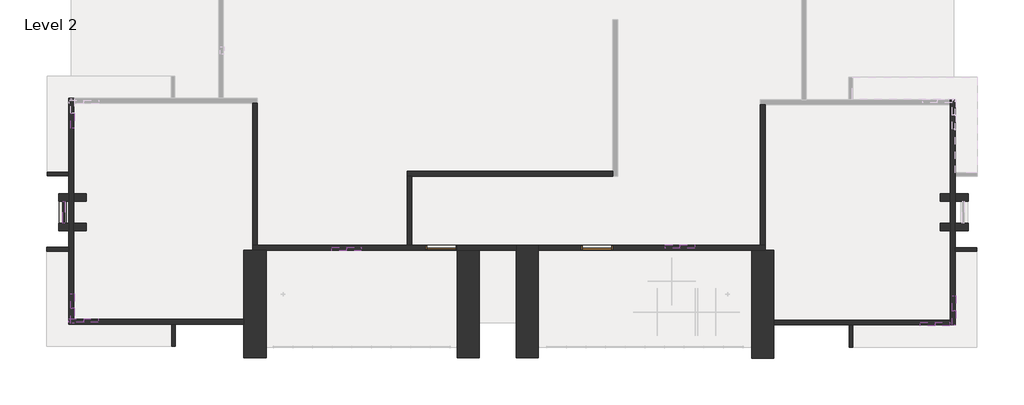
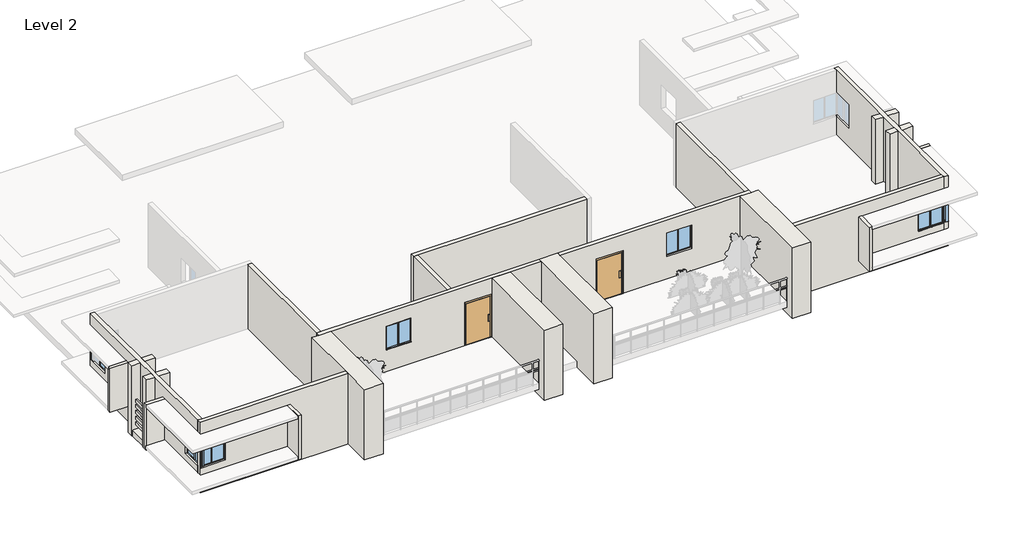
# One storey, part 1 of 4: 39 walls, 13 windows, 2 doors.
"""IFC4 building model written with IfcOpenShell, lengths in millimetres."""

from ifc_helpers import new_model, si_unit, frame, origin, place, context, project, spatial, polyline, outline, extrude, faceted_brep, transform, mapped, element, save
from components import door_15d3c954, window_20ff4747

model = new_model("IFC4")

# Units and contexts
model_context = context("Model", 3, world=origin())
ifc_project = project(units=[si_unit("LENGTHUNIT", "METRE", prefix="MILLI")], contexts=[model_context])

# Site, building, storey
site = spatial("IfcSite", under=ifc_project)
building = spatial("IfcBuilding", under=site)
storey = spatial("IfcBuildingStorey", under=building, Name="Level 2", Elevation=3048.0)

# Doors
placement = place(None, origin())
door_shape = door_15d3c954(model_context)
element("IfcDoor", 1, ObjectType="Door-Passage-Single-Flush-Dbl_Acting : 48\" x 96\"", at=placement, inside=storey, context=model_context, shape_type="MappedRepresentation", body=[
    mapped(door_shape, transform((7011.0520665, -5255.880811, 3657.6), x_axis=(-1.0, 0.0, 0.0), y_axis=(0.0, -1.0, 0.0), z_axis=(0.0, 0.0, 1.0))),
])
element("IfcDoor", 2, ObjectType="Door-Passage-Single-Flush-Dbl_Acting : 48\" x 96\"", at=placement, inside=storey, context=model_context, shape_type="MappedRepresentation", body=[
    mapped(door_shape, transform((559.4520665, -5255.1961695, 3657.6), x_axis=(-1.0, 0.0, 0.0), y_axis=(0.0, -1.0, 0.0), z_axis=(0.0, 0.0, 1.0))),
])

# Walls
element("IfcWall", 3, ObjectType="Generic - 1'", at=placement, inside=storey, context=model_context, shape_type="SweptSolid", body=[
    extrude(outline(polyline([(-14151.7972154, -3343.5294056), (-14680.5479335, -3343.5294056), (-14680.5479335, -3038.7294056), (-14151.7972154, -3038.7294056), (-14151.7972154, -3343.5294056)])), frame((0.0, 0.0, 3048.0), z_axis=(0.0, 0.0, 1.0), x_axis=(1.0, 0.0, 0.0)), (0.0, 0.0, 1.0), 3657.6),
])
element("IfcWall", 4, ObjectType="Generic - 1'", at=placement, inside=storey, context=model_context, shape_type="Brep", body=[
    faceted_brep([(-14883.7479335, -3038.7294056, 3048.0), (-15302.1394029, -3038.7294056, 3048.0), (-15302.1394029, -3038.7294056, 6705.6), (-14883.7479335, -3038.7294056, 6705.6), (-14883.7479335, -3343.5294056, 3048.0), (-14883.7479335, -3343.5294056, 6705.6), (-15302.1394029, -3343.5294056, 6705.6), (-15302.1394029, -3343.5294056, 3048.0), (-15277.0936682, -3343.5294056, 3048.0), (-14972.2936682, -3343.5294056, 3048.0)], [[[0, 1, 2, 3]], [[4, 5, 6, 7, 8, 9]], [[1, 0, 4, 9, 8, 7]], [[2, 1, 7, 6]], [[3, 2, 6, 5]], [[0, 3, 5, 4]]]),
])
element("IfcWall", 5, ObjectType="Generic - 1'", at=placement, inside=storey, context=model_context, shape_type="SweptSolid", body=[
    extrude(outline(polyline([(-14151.7972154, -4562.7294056), (-14680.5479335, -4562.7294056), (-14680.5479335, -4257.9294056), (-14151.7972154, -4257.9294056), (-14151.7972154, -4562.7294056)])), frame((0.0, 0.0, 3048.0), z_axis=(0.0, 0.0, 1.0), x_axis=(1.0, 0.0, 0.0)), (0.0, 0.0, 1.0), 3657.6),
])
element("IfcWall", 6, ObjectType="Generic - 1'", at=placement, inside=storey, context=model_context, shape_type="Brep", body=[
    faceted_brep([(-14883.7479335, -4257.9294056, 3048.0), (-14972.2936682, -4257.9294056, 3048.0), (-15277.0936682, -4257.9294056, 3048.0), (-15302.1394029, -4257.9294056, 3048.0), (-15302.1394029, -4257.9294056, 6705.6), (-14883.7479335, -4257.9294056, 6705.6), (-14883.7479335, -4562.7294056, 3048.0), (-14883.7479335, -4562.7294056, 6705.6), (-15302.1394029, -4562.7294056, 6705.6), (-15302.1394029, -4562.7294056, 3048.0)], [[[0, 1, 2, 3, 4, 5]], [[6, 7, 8, 9]], [[3, 2, 1, 0, 6, 9]], [[4, 3, 9, 8]], [[5, 4, 8, 7]], [[0, 5, 7, 6]]]),
])
element("IfcWall", 7, ObjectType="Generic - 1'", at=placement, inside=storey, context=model_context, shape_type="Brep", body=[
    faceted_brep([(21857.3520665, -3343.5294056, 3048.0), (22069.7857703, -3343.5294056, 3048.0), (22374.5857703, -3343.5294056, 3048.0), (22386.1027846, -3343.5294056, 3048.0), (22386.1027846, -3343.5294056, 6705.6), (21857.3520665, -3343.5294056, 6705.6), (21857.3520665, -3038.7294056, 3048.0), (21857.3520665, -3038.7294056, 6705.6), (22386.1027846, -3038.7294056, 6705.6), (22386.1027846, -3038.7294056, 3048.0)], [[[0, 1, 2, 3, 4, 5]], [[6, 7, 8, 9]], [[3, 2, 1, 0, 6, 9]], [[4, 3, 9, 8]], [[5, 4, 8, 7]], [[0, 5, 7, 6]]]),
])
element("IfcWall", 8, ObjectType="Generic - 1'", at=placement, inside=storey, context=model_context, shape_type="SweptSolid", body=[
    extrude(outline(polyline([(21235.7605971, -3038.7294056), (21654.1520665, -3038.7294056), (21654.1520665, -3343.5294056), (21235.7605971, -3343.5294056), (21235.7605971, -3038.7294056)])), frame((0.0, 0.0, 3048.0), z_axis=(0.0, 0.0, 1.0), x_axis=(1.0, 0.0, 0.0)), (0.0, 0.0, 1.0), 3657.6),
])
element("IfcWall", 9, ObjectType="Generic - 1'", at=placement, inside=storey, context=model_context, shape_type="Brep", body=[
    faceted_brep([(21857.3520665, -4562.7294056, 3048.0), (22386.1027846, -4562.7294056, 3048.0), (22386.1027846, -4562.7294056, 6705.6), (21857.3520665, -4562.7294056, 6705.6), (21857.3520665, -4257.9294056, 3048.0), (21857.3520665, -4257.9294056, 6705.6), (22386.1027846, -4257.9294056, 6705.6), (22386.1027846, -4257.9294056, 3048.0), (22374.5857703, -4257.9294056, 3048.0), (22069.7857703, -4257.9294056, 3048.0)], [[[0, 1, 2, 3]], [[4, 5, 6, 7, 8, 9]], [[1, 0, 4, 9, 8, 7]], [[2, 1, 7, 6]], [[3, 2, 6, 5]], [[0, 3, 5, 4]]]),
])
element("IfcWall", 10, ObjectType="Generic - 1'", at=placement, inside=storey, context=model_context, shape_type="SweptSolid", body=[
    extrude(outline(polyline([(21235.7605971, -4257.9294056), (21654.1520665, -4257.9294056), (21654.1520665, -4562.7294056), (21235.7605971, -4562.7294056), (21235.7605971, -4257.9294056)])), frame((0.0, 0.0, 3048.0), z_axis=(0.0, 0.0, 1.0), x_axis=(1.0, 0.0, 0.0)), (0.0, 0.0, 1.0), 3657.6),
])
element("IfcWall", 11, ObjectType="Generic - 2'", at=placement, inside=storey, context=model_context, shape_type="SweptSolid", body=[
    extrude(outline(polyline([(-15277.0936682, -4257.9294056), (-15277.0936682, -3343.5294056), (-14972.2936682, -3343.5294056), (-14972.2936682, -4257.9294056), (-15277.0936682, -4257.9294056)])), frame((0.0, 0.0, 3048.0), z_axis=(0.0, 0.0, 1.0), x_axis=(1.0, 0.0, 0.0)), (0.0, 0.0, 1.0), 304.8),
])
element("IfcWall", 12, ObjectType="Generic - 3'", at=placement, inside=storey, context=model_context, shape_type="SweptSolid", body=[
    extrude(outline(polyline([(2134.2520665, -5363.1461695), (2134.2520665, -9833.5461695), (1219.8520665, -9833.5461695), (1219.8520665, -5363.1461695), (2134.2520665, -5363.1461695)])), frame((0.0, 0.0, 3048.0), z_axis=(0.0, 0.0, 1.0), x_axis=(1.0, 0.0, 0.0)), (0.0, 0.0, 1.0), 3657.6),
])
element("IfcWall", 13, ObjectType="Generic - 3'", at=placement, inside=storey, context=model_context, shape_type="Brep", body=[
    faceted_brep([(4572.6520665, -9833.5461695, 3048.0), (4572.6520665, -5363.830811, 3048.0), (4572.6520665, -5160.630811, 3048.0), (4572.6520665, -5160.630811, 6705.6), (4572.6520665, -5363.830811, 6705.6), (4572.6520665, -9833.5461695, 6705.6), (3658.2520665, -9833.5461695, 3048.0), (3658.2520665, -9833.5461695, 6705.6), (3658.2520665, -5363.1461695, 6705.6), (3658.2520665, -5160.630811, 6705.6), (3658.2520665, -5160.630811, 3048.0), (3658.2520665, -5363.1461695, 3048.0)], [[[0, 1, 2, 3, 4, 5]], [[6, 7, 8, 9, 10, 11]], [[2, 1, 0, 6, 11, 10]], [[5, 4, 3, 9, 8, 7]], [[0, 5, 7, 6]], [[3, 2, 10, 9]]]),
])
element("IfcWall", 14, ObjectType="Generic - 3'", at=placement, inside=storey, context=model_context, shape_type="Brep", body=[
    faceted_brep([(-7619.3479335, -5363.1461695, 3048.0), (-7619.3479335, -8237.0604699, 3048.0), (-7619.3479335, -8440.2604699, 3048.0), (-7619.3479335, -9833.5461695, 3048.0), (-7619.3479335, -9833.5461695, 6705.6), (-7619.3479335, -8440.2604699, 6705.6), (-7619.3479335, -8237.0604699, 6705.6), (-7619.3479335, -5363.1461695, 6705.6), (-6704.9479335, -5363.1461695, 3048.0), (-6704.9479335, -5363.1461695, 6705.6), (-6704.9479335, -9833.5461695, 6705.6), (-6704.9479335, -9833.5461695, 3048.0), (-7263.7479335, -5363.1461695, 3048.0), (-7263.7479335, -5363.1461695, 6705.6)], [[[0, 1, 2, 3, 4, 5, 6, 7]], [[8, 9, 10, 11]], [[3, 2, 1, 0, 12, 8, 11]], [[4, 3, 11, 10]], [[7, 6, 5, 4, 10, 9, 13]], [[0, 7, 13, 9, 8, 12]]]),
])
element("IfcWall", 15, ObjectType="Generic - 3'", at=placement, inside=storey, context=model_context, shape_type="Brep", body=[
    faceted_brep([(13411.8520665, -5363.830811, 3048.0), (13411.8520665, -9834.230811, 3048.0), (13411.8520665, -9834.230811, 6705.6), (13411.8520665, -5363.830811, 6705.6), (14326.2520665, -5363.830811, 3048.0), (14326.2520665, -5363.830811, 6705.6), (14326.2520665, -8263.1451114, 6705.6), (14326.2520665, -8466.3451114, 6705.6), (14326.2520665, -9834.230811, 6705.6), (14326.2520665, -9834.230811, 3048.0), (14326.2520665, -8466.3451114, 3048.0), (14326.2520665, -8263.1451114, 3048.0), (13970.6520665, -5363.830811, 3048.0), (13970.6520665, -5363.830811, 6705.6)], [[[0, 1, 2, 3]], [[4, 5, 6, 7, 8, 9, 10, 11]], [[1, 0, 12, 4, 11, 10, 9]], [[2, 1, 9, 8]], [[3, 2, 8, 7, 6, 5, 13]], [[0, 3, 13, 5, 4, 12]]]),
])
element("IfcWall", 16, ObjectType="Generic - 5\"", at=placement, inside=storey, context=model_context, shape_type="SweptSolid", body=[
    extrude(outline(polyline([(-15124.6936682, -4257.9294056), (-15124.6936682, -3343.5294056), (-15048.4936682, -3343.5294056), (-15048.4936682, -4257.9294056), (-15124.6936682, -4257.9294056)])), frame((0.0, 0.0, 3581.4), z_axis=(0.0, 0.0, 1.0), x_axis=(1.0, 0.0, 0.0)), (0.0, 0.0, 1.0), 152.8735856),
])
element("IfcWall", 17, ObjectType="Generic - 5\"", at=placement, inside=storey, context=model_context, shape_type="SweptSolid", body=[
    extrude(outline(polyline([(-15124.6936682, -4257.9294056), (-15124.6936682, -3343.5294056), (-15048.4936682, -3343.5294056), (-15048.4936682, -4257.9294056), (-15124.6936682, -4257.9294056)])), frame((0.0, 0.0, 3860.8), z_axis=(0.0, 0.0, 1.0), x_axis=(1.0, 0.0, 0.0)), (0.0, 0.0, 1.0), 152.8735856),
])
element("IfcWall", 18, ObjectType="Generic - 5\"", at=placement, inside=storey, context=model_context, shape_type="SweptSolid", body=[
    extrude(outline(polyline([(-15124.6936682, -4257.9294056), (-15124.6936682, -3343.5294056), (-15048.4936682, -3343.5294056), (-15048.4936682, -4257.9294056), (-15124.6936682, -4257.9294056)])), frame((0.0, 0.0, 4165.6), z_axis=(0.0, 0.0, 1.0), x_axis=(1.0, 0.0, 0.0)), (0.0, 0.0, 1.0), 152.8735856),
])
element("IfcWall", 19, ObjectType="Generic - 5\"", at=placement, inside=storey, context=model_context, shape_type="SweptSolid", body=[
    extrude(outline(polyline([(-15124.6936682, -4257.9294056), (-15124.6936682, -3343.5294056), (-15048.4936682, -3343.5294056), (-15048.4936682, -4257.9294056), (-15124.6936682, -4257.9294056)])), frame((0.0, 0.0, 4470.4), z_axis=(0.0, 0.0, 1.0), x_axis=(1.0, 0.0, 0.0)), (0.0, 0.0, 1.0), 152.8735856),
])
element("IfcWall", 20, ObjectType="Generic - 5\"", at=placement, inside=storey, context=model_context, shape_type="SweptSolid", body=[
    extrude(outline(polyline([(-15124.6936682, -4257.9294056), (-15124.6936682, -3343.5294056), (-15048.4936682, -3343.5294056), (-15048.4936682, -4257.9294056), (-15124.6936682, -4257.9294056)])), frame((0.0, 0.0, 4749.8), z_axis=(0.0, 0.0, 1.0), x_axis=(1.0, 0.0, 0.0)), (0.0, 0.0, 1.0), 152.8735856),
])
element("IfcWall", 21, ObjectType="Generic - 5\"", at=placement, inside=storey, context=model_context, shape_type="SweptSolid", body=[
    extrude(outline(polyline([(-15124.6936682, -4257.9294056), (-15124.6936682, -3343.5294056), (-15048.4936682, -3343.5294056), (-15048.4936682, -4257.9294056), (-15124.6936682, -4257.9294056)])), frame((0.0, 0.0, 3581.4), z_axis=(0.0, 0.0, 1.0), x_axis=(1.0, 0.0, 0.0)), (0.0, 0.0, 1.0), 152.8735856),
])
element("IfcWall", 22, ObjectType="Generic - 5\"", at=placement, inside=storey, context=model_context, shape_type="SweptSolid", body=[
    extrude(outline(polyline([(-15124.6936682, -4257.9294056), (-15124.6936682, -3343.5294056), (-15048.4936682, -3343.5294056), (-15048.4936682, -4257.9294056), (-15124.6936682, -4257.9294056)])), frame((0.0, 0.0, 3860.8), z_axis=(0.0, 0.0, 1.0), x_axis=(1.0, 0.0, 0.0)), (0.0, 0.0, 1.0), 152.8735856),
])
element("IfcWall", 23, ObjectType="Generic - 5\"", at=placement, inside=storey, context=model_context, shape_type="SweptSolid", body=[
    extrude(outline(polyline([(-15124.6936682, -4257.9294056), (-15124.6936682, -3343.5294056), (-15048.4936682, -3343.5294056), (-15048.4936682, -4257.9294056), (-15124.6936682, -4257.9294056)])), frame((0.0, 0.0, 4165.6), z_axis=(0.0, 0.0, 1.0), x_axis=(1.0, 0.0, 0.0)), (0.0, 0.0, 1.0), 152.8735856),
])
element("IfcWall", 24, ObjectType="Generic - 5\"", at=placement, inside=storey, context=model_context, shape_type="SweptSolid", body=[
    extrude(outline(polyline([(-15124.6936682, -4257.9294056), (-15124.6936682, -3343.5294056), (-15048.4936682, -3343.5294056), (-15048.4936682, -4257.9294056), (-15124.6936682, -4257.9294056)])), frame((0.0, 0.0, 4470.4), z_axis=(0.0, 0.0, 1.0), x_axis=(1.0, 0.0, 0.0)), (0.0, 0.0, 1.0), 152.8735856),
])
element("IfcWall", 25, ObjectType="Generic - 5\"", at=placement, inside=storey, context=model_context, shape_type="SweptSolid", body=[
    extrude(outline(polyline([(-15124.6936682, -4257.9294056), (-15124.6936682, -3343.5294056), (-15048.4936682, -3343.5294056), (-15048.4936682, -4257.9294056), (-15124.6936682, -4257.9294056)])), frame((0.0, 0.0, 4749.8), z_axis=(0.0, 0.0, 1.0), x_axis=(1.0, 0.0, 0.0)), (0.0, 0.0, 1.0), 152.8735856),
])
element("IfcWall", 26, ObjectType="Generic - 5\"", at=placement, inside=storey, context=model_context, shape_type="SweptSolid", body=[
    extrude(outline(polyline([(22145.9857703, -4257.9294056), (22145.9857703, -3343.5294056), (22222.1857703, -3343.5294056), (22222.1857703, -4257.9294056), (22145.9857703, -4257.9294056)])), frame((0.0, 0.0, 3581.4), z_axis=(0.0, 0.0, 1.0), x_axis=(1.0, 0.0, 0.0)), (0.0, 0.0, 1.0), 152.8735856),
])
element("IfcWall", 27, ObjectType="Generic - 6\"", at=placement, inside=storey, context=model_context, shape_type="SweptSolid", body=[
    extrude(outline(polyline([(22749.4138484, -5418.3451114), (21857.3520665, -5418.3451114), (21857.3520665, -5265.9451114), (22749.4138484, -5265.9451114), (22749.4138484, -5418.3451114)])), frame((0.0, 0.0, 3810.0), z_axis=(0.0, 0.0, 1.0), x_axis=(1.0, 0.0, 0.0)), (0.0, 0.0, 1.0), 2286.0),
])
element("IfcWall", 28, ObjectType="Generic - 6\"", at=placement, inside=storey, context=model_context, shape_type="SweptSolid", body=[
    extrude(outline(polyline([(17454.3075984, -9380.7451114), (17454.3075984, -8466.3451114), (17606.7075984, -8466.3451114), (17606.7075984, -9380.7451114), (17454.3075984, -9380.7451114)])), frame((0.0, 0.0, 3810.0), z_axis=(0.0, 0.0, 1.0), x_axis=(1.0, 0.0, 0.0)), (0.0, 0.0, 1.0), 2286.0),
])
element("IfcWall", 29, ObjectType="Generic - 6\"", at=placement, inside=storey, context=model_context, shape_type="SweptSolid", body=[
    extrude(outline(polyline([(-15775.8097154, -2128.3604699), (-14883.7479335, -2128.3604699), (-14883.7479335, -2280.7604699), (-15775.8097154, -2280.7604699), (-15775.8097154, -2128.3604699)])), frame((0.0, 0.0, 3810.0), z_axis=(0.0, 0.0, 1.0), x_axis=(1.0, 0.0, 0.0)), (0.0, 0.0, 1.0), 2286.0),
])
element("IfcWall", 30, ObjectType="Generic - 6\"", at=placement, inside=storey, context=model_context, shape_type="SweptSolid", body=[
    extrude(outline(polyline([(-15796.5604335, -5250.9729699), (-14883.7479335, -5250.9729699), (-14883.7479335, -5403.3729699), (-15796.5604335, -5403.3729699), (-15796.5604335, -5250.9729699)])), frame((0.0, 0.0, 3810.0), z_axis=(0.0, 0.0, 1.0), x_axis=(1.0, 0.0, 0.0)), (0.0, 0.0, 1.0), 2286.0),
])
element("IfcWall", 31, ObjectType="Generic - 6\"", at=placement, inside=storey, context=model_context, shape_type="SweptSolid", body=[
    extrude(outline(polyline([(-10607.7034654, -9354.6604699), (-10607.7034654, -8440.2604699), (-10455.3034654, -8440.2604699), (-10455.3034654, -9354.6604699), (-10607.7034654, -9354.6604699)])), frame((0.0, 0.0, 3810.0), z_axis=(0.0, 0.0, 1.0), x_axis=(1.0, 0.0, 0.0)), (0.0, 0.0, 1.0), 2286.0),
])
element("IfcWall", 32, ObjectType="Generic - 8\"", at=placement, inside=storey, context=model_context, shape_type="Brep", body=[
    faceted_brep([(7671.4520665, -2102.9604699, 3657.6), (-862.9479335, -2102.9604699, 3657.6), (-862.9479335, -2102.9604699, 6705.6), (7671.4520665, -2102.9604699, 6705.6), (7671.4520665, -2306.1604699, 3657.6), (7671.4520665, -2306.1604699, 6705.6), (-659.7479335, -2306.1604699, 6705.6), (-862.9479335, -2306.1604699, 6705.6), (-862.9479335, -2306.1604699, 3657.6), (-659.7479335, -2306.1604699, 3657.6)], [[[0, 1, 2, 3]], [[4, 5, 6, 7, 8, 9]], [[1, 0, 4, 9, 8]], [[3, 2, 7, 6, 5]], [[0, 3, 5, 4]], [[2, 1, 8, 7]]]),
])
element("IfcWall", 33, ObjectType="Generic - 8\"", at=placement, inside=storey, context=model_context, shape_type="SweptSolid", body=[
    extrude(outline(polyline([(-862.9479335, -5159.9461695), (-862.9479335, -2306.1604699), (-659.7479335, -2306.1604699), (-659.7479335, -5159.9461695), (-862.9479335, -5159.9461695)])), frame((0.0, 0.0, 3657.6), z_axis=(0.0, 0.0, 1.0), x_axis=(1.0, 0.0, 0.0)), (0.0, 0.0, 1.0), 3048.0),
])
element("IfcWall", 34, ObjectType="Generic - 8\" gray", at=placement, inside=storey, context=model_context, shape_type="Brep", body=[
    faceted_brep([(-14883.7479335, -8440.2604699, 3048.0), (-7619.3479335, -8440.2604699, 3048.0), (-7619.3479335, -8440.2604699, 6705.6), (-14883.7479335, -8440.2604699, 6705.6), (-13655.3509584, -8440.2604699, 4320.2804451), (-14874.5509584, -8440.2604699, 4320.2804451), (-14874.5509584, -8440.2604699, 5539.4804451), (-13655.3509584, -8440.2604699, 5539.4804451), (-7619.3479335, -8237.0604699, 3048.0), (-14680.5479335, -8237.0604699, 3048.0), (-14883.7479335, -8237.0604699, 3048.0), (-14883.7479335, -8237.0604699, 4320.2804451), (-14883.7479335, -8237.0604699, 5539.4804451), (-14883.7479335, -8237.0604699, 6705.6), (-14680.5479335, -8237.0604699, 6705.6), (-7619.3479335, -8237.0604699, 6705.6), (-14874.5509584, -8237.0604699, 4320.2804451), (-14680.5479335, -8237.0604699, 4320.2804451), (-13655.3509584, -8237.0604699, 4320.2804451), (-13655.3509584, -8237.0604699, 5539.4804451), (-14680.5479335, -8237.0604699, 5539.4804451), (-14874.5509584, -8237.0604699, 5539.4804451)], [[[0, 1, 2, 3], [4, 5, 6, 7]], [[8, 9, 10, 11, 12, 13, 14, 15], [16, 17, 18, 19, 20, 21]], [[1, 0, 10, 9, 8]], [[3, 2, 15, 14, 13]], [[0, 3, 13, 12, 11, 10]], [[2, 1, 8, 15]], [[4, 18, 17, 16, 5]], [[6, 5, 16, 21]], [[6, 21, 20, 19, 7]], [[7, 19, 18, 4]]]),
])
element("IfcWall", 35, ObjectType="Generic - 8\" gray", at=placement, inside=storey, context=model_context, shape_type="Brep", body=[
    faceted_brep([(-14883.7479335, 919.6395301, 3048.0), (-14883.7479335, -3038.7294056, 3048.0), (-14883.7479335, -3343.5294056, 3048.0), (-14883.7479335, -4257.9294056, 3048.0), (-14883.7479335, -4562.7294056, 3048.0), (-14883.7479335, -8237.0604699, 3048.0), (-14883.7479335, -8237.0604699, 4320.2804451), (-14883.7479335, -7169.263768, 4320.2804451), (-14883.7479335, -7169.263768, 5539.4804451), (-14883.7479335, -8237.0604699, 5539.4804451), (-14883.7479335, -8237.0604699, 6705.6), (-14883.7479335, -4562.7294056, 6705.6), (-14883.7479335, -4257.9294056, 6705.6), (-14883.7479335, -3343.5294056, 6705.6), (-14883.7479335, -3038.7294056, 6705.6), (-14883.7479335, 919.6395301, 6705.6), (-14883.7479335, -310.2864811, 4320.2804451), (-14883.7479335, 908.9135189, 4320.2804451), (-14883.7479335, 908.9135189, 5539.4804451), (-14883.7479335, -310.2864811, 5539.4804451), (-14680.5479335, -8237.0604699, 3048.0), (-14680.5479335, -4562.7294056, 3048.0), (-14680.5479335, -4257.9294056, 3048.0), (-14680.5479335, -3343.5294056, 3048.0), (-14680.5479335, -3038.7294056, 3048.0), (-14680.5479335, 716.4395301, 3048.0), (-14680.5479335, 919.6395301, 3048.0), (-14680.5479335, 919.6395301, 4320.2804451), (-14680.5479335, 919.6395301, 5539.4804451), (-14680.5479335, 919.6395301, 6705.6), (-14680.5479335, 716.4395301, 6705.6), (-14680.5479335, -3038.7294056, 6705.6), (-14680.5479335, -3343.5294056, 6705.6), (-14680.5479335, -4257.9294056, 6705.6), (-14680.5479335, -4562.7294056, 6705.6), (-14680.5479335, -8237.0604699, 6705.6), (-14680.5479335, -8237.0604699, 5539.4804451), (-14680.5479335, -7169.263768, 5539.4804451), (-14680.5479335, -7169.263768, 4320.2804451), (-14680.5479335, -8237.0604699, 4320.2804451), (-14680.5479335, 908.9135189, 4320.2804451), (-14680.5479335, 716.4395301, 4320.2804451), (-14680.5479335, -310.2864811, 4320.2804451), (-14680.5479335, -310.2864811, 5539.4804451), (-14680.5479335, 716.4395301, 5539.4804451), (-14680.5479335, 908.9135189, 5539.4804451), (-14874.5509584, -8237.0604699, 4320.2804451), (-14874.5509584, -8237.0604699, 5539.4804451)], [[[0, 1, 2, 3, 4, 5, 6, 7, 8, 9, 10, 11, 12, 13, 14, 15], [16, 17, 18, 19]], [[20, 21, 22, 23, 24, 25, 26, 27, 28, 29, 30, 31, 32, 33, 34, 35, 36, 37, 38, 39], [40, 41, 42, 43, 44, 45]], [[5, 4, 3, 2, 1, 0, 26, 25, 24, 23, 22, 21, 20]], [[15, 14, 13, 12, 11, 10, 35, 34, 33, 32, 31, 30, 29]], [[0, 15, 29, 28, 27, 26]], [[5, 20, 39, 46, 6]], [[35, 10, 9, 47, 36]], [[38, 7, 6, 46, 39]], [[8, 7, 38, 37]], [[8, 37, 36, 47, 9]], [[16, 42, 41, 40, 17]], [[18, 45, 44, 43, 19]], [[19, 43, 42, 16]], [[45, 18, 17, 40]]]),
])
element("IfcWall", 36, ObjectType="Generic - 8\" gray", at=placement, inside=storey, context=model_context, shape_type="Brep", body=[
    faceted_brep([(21654.1520665, 868.1548886, 3048.0), (21654.1520665, 664.9548886, 3048.0), (21654.1520665, -3038.7294056, 3048.0), (21654.1520665, -3343.5294056, 3048.0), (21654.1520665, -4257.9294056, 3048.0), (21654.1520665, -4562.7294056, 3048.0), (21654.1520665, -8263.1451114, 3048.0), (21654.1520665, -8466.3451114, 3048.0), (21654.1520665, -8466.3451114, 4320.2804451), (21654.1520665, -7262.9130582, 4320.2804451), (21654.1520665, -7262.9130582, 5539.4804451), (21654.1520665, -8466.3451114, 5539.4804451), (21654.1520665, -8466.3451114, 6705.6), (21654.1520665, -8263.1451114, 6705.6), (21654.1520665, -4562.7294056, 6705.6), (21654.1520665, -4257.9294056, 6705.6), (21654.1520665, -3343.5294056, 6705.6), (21654.1520665, -3038.7294056, 6705.6), (21654.1520665, 664.9548886, 6705.6), (21654.1520665, 868.1548886, 6705.6), (21654.1520665, 868.1548886, 5539.4804451), (21654.1520665, 868.1548886, 4320.2804451), (21654.1520665, 859.364485, 4320.2804451), (21654.1520665, 859.364485, 5539.4804451), (21654.1520665, 664.9548886, 5539.4804451), (21654.1520665, -359.835515, 5539.4804451), (21654.1520665, -359.835515, 4320.2804451), (21654.1520665, 664.9548886, 4320.2804451), (21857.3520665, -8466.3451114, 3048.0), (21857.3520665, -4562.7294056, 3048.0), (21857.3520665, -4257.9294056, 3048.0), (21857.3520665, -3343.5294056, 3048.0), (21857.3520665, -3038.7294056, 3048.0), (21857.3520665, 868.1548886, 3048.0), (21857.3520665, 868.1548886, 6705.6), (21857.3520665, -3038.7294056, 6705.6), (21857.3520665, -3343.5294056, 6705.6), (21857.3520665, -4257.9294056, 6705.6), (21857.3520665, -4562.7294056, 6705.6), (21857.3520665, -8466.3451114, 6705.6), (21857.3520665, -8466.3451114, 5539.4804451), (21857.3520665, -7262.9130582, 5539.4804451), (21857.3520665, -7262.9130582, 4320.2804451), (21857.3520665, -8466.3451114, 4320.2804451), (21857.3520665, 859.364485, 5539.4804451), (21857.3520665, 859.364485, 4320.2804451), (21857.3520665, -359.835515, 4320.2804451), (21857.3520665, -359.835515, 5539.4804451)], [[[0, 1, 2, 3, 4, 5, 6, 7, 8, 9, 10, 11, 12, 13, 14, 15, 16, 17, 18, 19, 20, 21], [22, 23, 24, 25, 26, 27]], [[28, 29, 30, 31, 32, 33, 34, 35, 36, 37, 38, 39, 40, 41, 42, 43], [44, 45, 46, 47]], [[7, 6, 5, 4, 3, 2, 1, 0, 33, 32, 31, 30, 29, 28]], [[19, 18, 17, 16, 15, 14, 13, 12, 39, 38, 37, 36, 35, 34]], [[0, 21, 20, 19, 34, 33]], [[7, 28, 43, 8]], [[39, 12, 11, 40]], [[45, 22, 27, 26, 46]], [[23, 22, 45, 44]], [[23, 44, 47, 25, 24]], [[25, 47, 46, 26]], [[8, 43, 42, 9]], [[10, 9, 42, 41]], [[10, 41, 40, 11]]]),
])
element("IfcWall", 37, ObjectType="Generic - 8\" gray", at=placement, inside=storey, context=model_context, shape_type="Brep", body=[
    faceted_brep([(3658.2520665, -5159.9461695, 3048.0), (-7060.5479335, -5159.9461695, 3048.0), (-7263.7479335, -5159.9461695, 3048.0), (-7263.7479335, -5159.9461695, 6705.6), (-7060.5479335, -5159.9461695, 6705.6), (-862.9479335, -5159.9461695, 6705.6), (-659.7479335, -5159.9461695, 6705.6), (3658.2520665, -5159.9461695, 6705.6), (-2753.0651847, -5159.9461695, 4797.0951112), (-2753.0651847, -5159.9461695, 6016.2951112), (-3972.2651847, -5159.9461695, 6016.2951112), (-3972.2651847, -5159.9461695, 4797.0951112), (-100.9479335, -5159.9461695, 5892.8), (-100.9479335, -5159.9461695, 3657.6), (1219.8520665, -5159.9461695, 3657.6), (1219.8520665, -5159.9461695, 5892.8), (-7263.7479335, -5363.1461695, 3048.0), (-6704.9479335, -5363.1461695, 3048.0), (1219.8520665, -5363.1461695, 3048.0), (2134.2520665, -5363.1461695, 3048.0), (3658.2520665, -5363.1461695, 3048.0), (3658.2520665, -5363.1461695, 6705.6), (2134.2520665, -5363.1461695, 6705.6), (1219.8520665, -5363.1461695, 6705.6), (-6704.9479335, -5363.1461695, 6705.6), (-7263.7479335, -5363.1461695, 6705.6), (-2753.0651847, -5363.1461695, 6016.2951112), (-2753.0651847, -5363.1461695, 4797.0951112), (-3972.2651847, -5363.1461695, 4797.0951112), (-3972.2651847, -5363.1461695, 6016.2951112), (-100.9479335, -5363.1461695, 3657.6), (-100.9479335, -5363.1461695, 5892.8), (1219.8520665, -5363.1461695, 5892.8), (1219.8520665, -5363.1461695, 3657.6), (3658.2520665, -5160.630811, 3048.0), (3658.2520665, -5160.630811, 6705.6)], [[[0, 1, 2, 3, 4, 5, 6, 7], [8, 9, 10, 11], [12, 13, 14, 15]], [[16, 17, 18, 19, 20, 21, 22, 23, 24, 25], [26, 27, 28, 29], [30, 31, 32, 33]], [[2, 1, 0, 34, 20, 19, 18, 17, 16]], [[7, 6, 5, 4, 3, 25, 24, 23, 22, 21, 35]], [[0, 7, 35, 21, 20, 34]], [[3, 2, 16, 25]], [[27, 8, 11, 28]], [[9, 8, 27, 26]], [[9, 26, 29, 10]], [[10, 29, 28, 11]], [[30, 13, 12, 31]], [[31, 12, 15, 32]], [[32, 15, 14, 33]], [[13, 30, 33, 14]]]),
])
element("IfcWall", 38, ObjectType="Generic - 8\" gray", at=placement, inside=storey, context=model_context, shape_type="Brep", body=[
    faceted_brep([(4572.6520665, -5363.830811, 3048.0), (13411.8520665, -5363.830811, 3048.0), (13970.6520665, -5363.830811, 3048.0), (13970.6520665, -5363.830811, 6705.6), (13411.8520665, -5363.830811, 6705.6), (4572.6520665, -5363.830811, 6705.6), (9831.9980014, -5363.830811, 4815.8493508), (9831.9980014, -5363.830811, 6035.0493508), (11051.1980014, -5363.830811, 6035.0493508), (11051.1980014, -5363.830811, 4815.8493508), (6350.6520665, -5363.830811, 3657.6), (6350.6520665, -5363.830811, 5892.8), (7671.4520665, -5363.830811, 5892.8), (7671.4520665, -5363.830811, 3657.6), (13970.6520665, -5160.630811, 3048.0), (13767.4520665, -5160.630811, 3048.0), (4572.6520665, -5160.630811, 3048.0), (4572.6520665, -5160.630811, 6705.6), (13767.4520665, -5160.630811, 6705.6), (13970.6520665, -5160.630811, 6705.6), (9831.9980014, -5160.630811, 6035.0493508), (9831.9980014, -5160.630811, 4815.8493508), (11051.1980014, -5160.630811, 4815.8493508), (11051.1980014, -5160.630811, 6035.0493508), (6350.6520665, -5160.630811, 5892.8), (6350.6520665, -5160.630811, 3657.6), (7671.4520665, -5160.630811, 3657.6), (7671.4520665, -5160.630811, 5892.8)], [[[0, 1, 2, 3, 4, 5], [6, 7, 8, 9], [10, 11, 12, 13]], [[14, 15, 16, 17, 18, 19], [20, 21, 22, 23], [24, 25, 26, 27]], [[2, 1, 0, 16, 15, 14]], [[5, 4, 3, 19, 18, 17]], [[0, 5, 17, 16]], [[3, 2, 14, 19]], [[21, 6, 9, 22]], [[7, 6, 21, 20]], [[7, 20, 23, 8]], [[8, 23, 22, 9]], [[10, 25, 24, 11]], [[11, 24, 27, 12]], [[12, 27, 26, 13]], [[25, 10, 13, 26]]]),
])
element("IfcWall", 39, ObjectType="Generic - 8\" gray", at=placement, inside=storey, context=model_context, shape_type="Brep", body=[
    faceted_brep([(21654.1520665, -8263.1451114, 3048.0), (14326.2520665, -8263.1451114, 3048.0), (14326.2520665, -8263.1451114, 6705.6), (21654.1520665, -8263.1451114, 6705.6), (20403.2295783, -8263.1451114, 4320.2804451), (21622.4295783, -8263.1451114, 4320.2804451), (21622.4295783, -8263.1451114, 5539.4804451), (20403.2295783, -8263.1451114, 5539.4804451), (14326.2520665, -8466.3451114, 3048.0), (21654.1520665, -8466.3451114, 3048.0), (21654.1520665, -8466.3451114, 4320.2804451), (21654.1520665, -8466.3451114, 5539.4804451), (21654.1520665, -8466.3451114, 6705.6), (14326.2520665, -8466.3451114, 6705.6), (21622.4295783, -8466.3451114, 4320.2804451), (20403.2295783, -8466.3451114, 4320.2804451), (20403.2295783, -8466.3451114, 5539.4804451), (21622.4295783, -8466.3451114, 5539.4804451)], [[[0, 1, 2, 3], [4, 5, 6, 7]], [[8, 9, 10, 11, 12, 13], [14, 15, 16, 17]], [[1, 0, 9, 8]], [[3, 2, 13, 12]], [[0, 3, 12, 11, 10, 9]], [[2, 1, 8, 13]], [[4, 15, 14, 5]], [[6, 5, 14, 17]], [[6, 17, 16, 7]], [[7, 16, 15, 4]]]),
])
element("IfcWall", 40, ObjectType="Generic - 8\" gray", at=placement, inside=storey, context=model_context, shape_type="SweptSolid", body=[
    extrude(outline(polyline([(-7263.7479335, -5159.9461695), (-7263.7479335, 716.4395301), (-7060.5479335, 716.4395301), (-7060.5479335, -5159.9461695), (-7263.7479335, -5159.9461695)])), frame((0.0, 0.0, 3048.0), z_axis=(0.0, 0.0, 1.0), x_axis=(1.0, 0.0, 0.0)), (0.0, 0.0, 1.0), 3657.6),
])
element("IfcWall", 41, ObjectType="Generic - 8\" gray", at=placement, inside=storey, context=model_context, shape_type="SweptSolid", body=[
    extrude(outline(polyline([(13767.4520665, -5160.630811), (13767.4520665, 664.9548886), (13970.6520665, 664.9548886), (13970.6520665, -5160.630811), (13767.4520665, -5160.630811)])), frame((0.0, 0.0, 3048.0), z_axis=(0.0, 0.0, 1.0), x_axis=(1.0, 0.0, 0.0)), (0.0, 0.0, 1.0), 3657.6),
])

# Windows
window_shape = window_20ff4747(model_context)
element("IfcWindow", 42, ObjectType="Instance - Fixed : 24\" x 48\"", at=placement, inside=storey, context=model_context, shape_type="MappedRepresentation", body=[
    mapped(window_shape, transform((21755.7520665, -8215.4130582, 3405.8804451), x_axis=(0.0, -1.0, 0.0), y_axis=(1.0, 0.0, 0.0), z_axis=(0.0, 0.0, 1.0))),
])
element("IfcWindow", 43, ObjectType="Instance - Fixed : 24\" x 48\"", at=placement, inside=storey, context=model_context, shape_type="MappedRepresentation", body=[
    mapped(window_shape, transform((21755.7520665, -7605.8130582, 3405.8804451), x_axis=(0.0, -1.0, 0.0), y_axis=(1.0, 0.0, 0.0), z_axis=(0.0, 0.0, 1.0))),
])
element("IfcWindow", 44, ObjectType="Instance - Fixed : 24\" x 48\"", at=placement, inside=storey, context=model_context, shape_type="MappedRepresentation", body=[
    mapped(window_shape, transform((20669.9295783, -8364.7451114, 3405.8804451), x_axis=(-1.0, 0.0, 0.0), y_axis=(0.0, -1.0, 0.0), z_axis=(0.0, 0.0, 1.0))),
])
element("IfcWindow", 45, ObjectType="Instance - Fixed : 24\" x 48\"", at=placement, inside=storey, context=model_context, shape_type="MappedRepresentation", body=[
    mapped(window_shape, transform((21279.5295783, -8364.7451114, 3405.8804451), x_axis=(-1.0, 0.0, 0.0), y_axis=(0.0, -1.0, 0.0), z_axis=(0.0, 0.0, 1.0))),
])
element("IfcWindow", 46, ObjectType="Instance - Fixed : 24\" x 48\"", at=placement, inside=storey, context=model_context, shape_type="MappedRepresentation", body=[
    mapped(window_shape, transform((-13922.0509584, -8338.6604699, 3405.8804451), x_axis=(1.0, 0.0, 0.0), y_axis=(0.0, 1.0, 0.0), z_axis=(0.0, 0.0, 1.0))),
])
element("IfcWindow", 47, ObjectType="Instance - Fixed : 24\" x 48\"", at=placement, inside=storey, context=model_context, shape_type="MappedRepresentation", body=[
    mapped(window_shape, transform((-14531.6509584, -8338.6604699, 3405.8804451), x_axis=(1.0, 0.0, 0.0), y_axis=(0.0, 1.0, 0.0), z_axis=(0.0, 0.0, 1.0))),
])
element("IfcWindow", 48, ObjectType="Instance - Fixed : 24\" x 48\"", at=placement, inside=storey, context=model_context, shape_type="MappedRepresentation", body=[
    mapped(window_shape, transform((-14782.1479335, -8121.763768, 3405.8804451), x_axis=(0.0, -1.0, 0.0), y_axis=(1.0, 0.0, 0.0), z_axis=(0.0, 0.0, 1.0))),
])
element("IfcWindow", 49, ObjectType="Instance - Fixed : 24\" x 48\"", at=placement, inside=storey, context=model_context, shape_type="MappedRepresentation", body=[
    mapped(window_shape, transform((-14782.1479335, -7512.163768, 3405.8804451), x_axis=(0.0, -1.0, 0.0), y_axis=(1.0, 0.0, 0.0), z_axis=(0.0, 0.0, 1.0))),
])
element("IfcWindow", 50, ObjectType="Instance - Fixed : 24\" x 48\"", at=placement, inside=storey, context=model_context, shape_type="MappedRepresentation", body=[
    mapped(window_shape, transform((-14782.1479335, -43.5864811, 3405.8804451), x_axis=(0.0, -1.0, 0.0), y_axis=(1.0, 0.0, 0.0), z_axis=(0.0, 0.0, 1.0))),
])
element("IfcWindow", 51, ObjectType="Instance - Fixed : 24\" x 48\"", at=placement, inside=storey, context=model_context, shape_type="MappedRepresentation", body=[
    mapped(window_shape, transform((-3705.5651847, -5261.5461695, 3882.6951112), x_axis=(-1.0, 0.0, 0.0), y_axis=(0.0, -1.0, 0.0), z_axis=(0.0, 0.0, 1.0))),
])
element("IfcWindow", 52, ObjectType="Instance - Fixed : 24\" x 48\"", at=placement, inside=storey, context=model_context, shape_type="MappedRepresentation", body=[
    mapped(window_shape, transform((-3095.9651847, -5261.5461695, 3882.6951112), x_axis=(-1.0, 0.0, 0.0), y_axis=(0.0, -1.0, 0.0), z_axis=(0.0, 0.0, 1.0))),
])
element("IfcWindow", 53, ObjectType="Instance - Fixed : 24\" x 48\"", at=placement, inside=storey, context=model_context, shape_type="MappedRepresentation", body=[
    mapped(window_shape, transform((10784.4980014, -5262.230811, 3901.4493508), x_axis=(1.0, 0.0, 0.0), y_axis=(0.0, 1.0, 0.0), z_axis=(0.0, 0.0, 1.0))),
])
element("IfcWindow", 54, ObjectType="Instance - Fixed : 24\" x 48\"", at=placement, inside=storey, context=model_context, shape_type="MappedRepresentation", body=[
    mapped(window_shape, transform((10174.8980014, -5262.230811, 3901.4493508), x_axis=(1.0, 0.0, 0.0), y_axis=(0.0, 1.0, 0.0), z_axis=(0.0, 0.0, 1.0))),
])

save(model, "model.ifc")

# Revit data of these elements
# Type "Door-Passage-Single-Flush-Dbl_Acting : 48\" x 96\""
#   Type Mark = "12"
#   Assembly Code = "B2030200"
#   Analytic Construction = "Wooden"
#   Thickness = 0' - 1 3/4"
#   Thermal Resistance (R) = 2.5876 (h·ft²·°F)/BTU
#   Swing Angle [instance default] = 45.00°
#   Strike Height = 3' - 4"
#   Rough Width [instance default] = 4' - 4"
#   Rough Height [instance default] = 7' - 4"
#   MF Opening Height [instance default] = 0' - 4"
#   MF Opening Width [instance default] = 0' - 4"
#   Inset Calculate [instance default] = 0' - 4"
#   Masonry Inset [instance default] = 0' - 1"
#   Height = 7' - 0"
#   Width = 4' - 0"
#   Heat Transfer Coefficient (U) = 0.3865 BTU/(h·ft²·°F)
#   Masonry Frame Depth = 0' - 5 3/4"
#   Masonry Frame [instance default] = yes
#   Function = 1
#   Dry Wall Frame [instance default] = no
#   Panel Material = Wood - Birch
#   Frame Material = Metal - Paint Finish - Grey
#   Door Handle Material = Aluminum
#   Visual Light Transmittance = 0
#   Solar Heat Gain Coefficient = 0
#   Wall Closure = (empty or 0)
# Type "Generic - 1'"
#   Assembly Code = "B2010"
#   Layers, outside or top first: 1' - 0" "Metal - Painted - Grey" (function 1)
# Type "Generic - 2'"
#   Assembly Code = "B2010"
#   Layers, outside or top first: 1' - 0" "Metal - Painted - Grey" (function 1)
# Type "Generic - 3'"
#   Assembly Code = "B2010"
#   Layers, outside or top first: 3' - 0" "Metal - Painted - Grey" (function 1)
# Type "Generic - 5\""
#   Assembly Code = "B2010"
#   Layers, outside or top first: 0' - 3" "Oak Flooring" (function 1)
# Type "Generic - 6\""
#   Assembly Code = "B2010"
#   Layers, outside or top first: 0' - 6" "Metal - Painted - Grey" (function 1)
# Type "Generic - 8\""
#   Assembly Code = "B2010"
#   Layers, outside or top first: 0' - 8" no material (function 1)
# Type "Generic - 8\" gray"
#   Assembly Code = "B2010"
#   Layers, outside or top first: 0' - 8" "Parking Stripe" (function 1)
# Type "Instance - Fixed : 24\" x 48\""
#   Type Mark = "11"
#   Construction Type Id = "GSP4R"
#   Assembly Code = "B2020100"
#   Analytic Construction = "1/8 in Pilkington single glazing"
#   Visual Light Transmittance = 0.9
#   Thermal Resistance (R) = 0.8466 (h·ft²·°F)/BTU
#   Solar Heat Gain Coefficient = 0.86
#   Heat Transfer Coefficient (U) = 1.1812 BTU/(h·ft²·°F)
#   Height [instance default] = 4' - 0"
#   Default Sill Height = 3' - 0"
#   Width [instance default] = 2' - 0"
#   Window Inset = 0' - 2"
#   Define Thermal Properties by = 1
#   Glass Pane Material = Glass
#   Sash Material = Iron, Ductile
#   Wall Closure = (empty or 0)
# Elements 1, 2 (IfcDoor, "Door-Passage-Single-Flush-Dbl_Acting : 48\" x 96\"")
#   Swing Angle = 45.00°
#   Rough Width = 4' - 4"
#   Rough Height = 7' - 4"
#   Masonry Inset = 0' - 1"
#   MF Opening Width = 0' - 4"
#   MF Opening Height = 0' - 4"
#   Inset Calculate = 0' - 4"
#   Masonry Frame = yes
#   Dry Wall Frame = no
#   Phase Created = New Construction
#   Materials on its faces: "Aluminum", "Metal - Paint Finish - Grey", "Wood - Birch"
# Elements 3, 4, 5, 6, 7, 8, 9, 10 (IfcWall, "Generic - 1'")
#   Top Offset = 0' - 0"
#   Base Offset = 0' - 0"
#   Unconnected Height = 12' - 0"
#   wall height = 12' - 0"
#   Phase Created = New Construction
#   Base Constraint = Level 2
#   Materials on its faces: "Metal - Painted - Grey"
# Element 11 (IfcWall, "Generic - 2'")
#   Top Offset = 0' - 0"
#   Base Offset = 0' - 0"
#   Unconnected Height = 1' - 0"
#   wall height = 1' - 0"
#   Phase Created = New Construction
#   Base Constraint = Level 2
#   Materials on its faces: "Metal - Painted - Grey"
# Elements 12, 14, 15 (IfcWall, "Generic - 3'")
#   Top Offset = 0' - 0"
#   Base Offset = 0' - 0"
#   Unconnected Height = 12' - 0"
#   wall height = 12' - 0"
#   Phase Created = New Construction
#   Base Constraint = Level 2
#   Materials on its faces: "Metal - Painted - Grey", "EIFS, Exterior Insulation"
# Element 13 (IfcWall, "Generic - 3'")
#   Top Offset = 0' - 0"
#   Base Offset = 0' - 0"
#   Unconnected Height = 12' - 0"
#   wall height = 12' - 0"
#   Phase Created = New Construction
#   Base Constraint = Level 2
#   Materials on its faces: "Metal - Painted - Grey", "Parking Stripe"
# Elements 16, 21, 26 (IfcWall, "Generic - 5\"")
#   built-in parameter 1001111 = 1' - 9"
#   Top Offset = -7' - 8.98135"
#   Base Offset = 1' - 9"
#   wall height = 0' - 6.01865"
#   Phase Created = New Construction
#   Base Constraint = Level 2
#   Top Constraint = Level 3
#   Materials on its faces: "Oak Flooring"
# Elements 17, 22 (IfcWall, "Generic - 5\"")
#   built-in parameter 1001111 = 2' - 8"
#   Top Offset = -6' - 9.98135"
#   Base Offset = 2' - 8"
#   wall height = 0' - 6.01865"
#   Phase Created = New Construction
#   Base Constraint = Level 2
#   Top Constraint = Level 3
#   Materials on its faces: "Oak Flooring"
# Elements 18, 23 (IfcWall, "Generic - 5\"")
#   built-in parameter 1001111 = 3' - 8"
#   Top Offset = -5' - 9.98135"
#   Base Offset = 3' - 8"
#   wall height = 0' - 6.01865"
#   Phase Created = New Construction
#   Base Constraint = Level 2
#   Top Constraint = Level 3
#   Materials on its faces: "Oak Flooring"
# Elements 19, 24 (IfcWall, "Generic - 5\"")
#   built-in parameter 1001111 = 4' - 8"
#   Top Offset = -4' - 9.98135"
#   Base Offset = 4' - 8"
#   wall height = 0' - 6.01865"
#   Phase Created = New Construction
#   Base Constraint = Level 2
#   Top Constraint = Level 3
#   Materials on its faces: "Oak Flooring"
# Elements 20, 25 (IfcWall, "Generic - 5\"")
#   built-in parameter 1001111 = 5' - 7"
#   Top Offset = -3' - 10.98135"
#   Base Offset = 5' - 7"
#   wall height = 0' - 6.01865"
#   Phase Created = New Construction
#   Base Constraint = Level 2
#   Top Constraint = Level 3
#   Materials on its faces: "Oak Flooring"
# Elements 27, 28, 29, 30, 31 (IfcWall, "Generic - 6\"")
#   built-in parameter 1001111 = 2' - 6"
#   Top Offset = 0' - 0"
#   Base Offset = 2' - 6"
#   Unconnected Height = 7' - 6"
#   wall height = 7' - 6"
#   Phase Created = New Construction
#   Base Constraint = Level 2
#   Materials on its faces: "Metal - Painted - Grey"
# Elements 32, 33 (IfcWall, "Generic - 8\"")
#   built-in parameter 1001111 = 2' - 0"
#   Top Offset = 0' - 0"
#   Base Offset = 2' - 0"
#   Unconnected Height = 10' - 0"
#   wall height = 10' - 0"
#   Phase Created = New Construction
#   Base Constraint = Level 2
#   Materials on its faces: "Default Wall"
# Element 34 (IfcWall, "Generic - 8\" gray")
#   Top Offset = 0' - 0"
#   Base Offset = 0' - 0"
#   Unconnected Height = 12' - 0"
#   wall height = 12' - 0"
#   Phase Created = New Construction
#   Base Constraint = Level 2
#   Materials on its faces: "Parking Stripe", "Rigid insulation", "EIFS, Exterior Insulation"
# Element 35 (IfcWall, "Generic - 8\" gray")
#   Top Offset = 0' - 0"
#   Base Offset = 0' - 0"
#   Unconnected Height = 12' - 0"
#   wall height = 12' - 0"
#   Phase Created = New Construction
#   Base Constraint = Level 2
#   Materials on its faces: "Parking Stripe", "EIFS, Exterior Insulation"
# Element 36 (IfcWall, "Generic - 8\" gray")
#   Top Offset = 0' - 0"
#   Base Offset = 0' - 0"
#   Unconnected Height = 12' - 0"
#   wall height = 12' - 0"
#   Phase Created = New Construction
#   Base Constraint = Level 2
#   Materials on its faces: "Parking Stripe", "EIFS, Exterior Insulation", "Rigid insulation"
# Elements 37, 38, 40, 41 (IfcWall, "Generic - 8\" gray")
#   Top Offset = 0' - 0"
#   Base Offset = 0' - 0"
#   Unconnected Height = 12' - 0"
#   wall height = 12' - 0"
#   Phase Created = New Construction
#   Base Constraint = Level 2
#   Materials on its faces: "Parking Stripe"
# Element 39 (IfcWall, "Generic - 8\" gray")
#   Top Offset = 0' - 0"
#   Base Offset = 0' - 0"
#   Unconnected Height = 12' - 0"
#   wall height = 12' - 0"
#   Phase Created = New Construction
#   Base Constraint = Level 2
#   Materials on its faces: "Parking Stripe", "Rigid insulation"
# Element 42 (IfcWindow, "Instance - Fixed : 24\" x 48\"")
#   Mark = "11"
#   Width = 2' - 0"
#   Height = 4' - 0"
#   Phase Created = New Construction
#   Materials on its faces: "Iron, Ductile", "Glass"
# Element 43 (IfcWindow, "Instance - Fixed : 24\" x 48\"")
#   Mark = "12"
#   Width = 2' - 0"
#   Height = 4' - 0"
#   Phase Created = New Construction
#   Materials on its faces: "Iron, Ductile", "Glass"
# Element 44 (IfcWindow, "Instance - Fixed : 24\" x 48\"")
#   Mark = "13"
#   Width = 2' - 0"
#   Height = 4' - 0"
#   Phase Created = New Construction
#   Materials on its faces: "Iron, Ductile", "Glass"
# Element 45 (IfcWindow, "Instance - Fixed : 24\" x 48\"")
#   Mark = "14"
#   Width = 2' - 0"
#   Height = 4' - 0"
#   Phase Created = New Construction
#   Materials on its faces: "Iron, Ductile", "Glass"
# Element 46 (IfcWindow, "Instance - Fixed : 24\" x 48\"")
#   Mark = "15"
#   Width = 2' - 0"
#   Height = 4' - 0"
#   Phase Created = New Construction
#   Materials on its faces: "Iron, Ductile", "Glass"
# Element 47 (IfcWindow, "Instance - Fixed : 24\" x 48\"")
#   Mark = "16"
#   Width = 2' - 0"
#   Height = 4' - 0"
#   Phase Created = New Construction
#   Materials on its faces: "Iron, Ductile", "Glass"
# Element 48 (IfcWindow, "Instance - Fixed : 24\" x 48\"")
#   Mark = "17"
#   Width = 2' - 0"
#   Height = 4' - 0"
#   Phase Created = New Construction
#   Materials on its faces: "Iron, Ductile", "Glass"
# Element 49 (IfcWindow, "Instance - Fixed : 24\" x 48\"")
#   Mark = "18"
#   Width = 2' - 0"
#   Height = 4' - 0"
#   Phase Created = New Construction
#   Materials on its faces: "Iron, Ductile", "Glass"
# Element 50 (IfcWindow, "Instance - Fixed : 24\" x 48\"")
#   Mark = "19"
#   Width = 2' - 0"
#   Height = 4' - 0"
#   Phase Created = New Construction
#   Materials on its faces: "Iron, Ductile", "Glass"
# Element 51 (IfcWindow, "Instance - Fixed : 24\" x 48\"")
#   Mark = "41"
#   Width = 2' - 0"
#   Height = 4' - 0"
#   Phase Created = New Construction
#   Materials on its faces: "Iron, Ductile", "Glass"
# Element 52 (IfcWindow, "Instance - Fixed : 24\" x 48\"")
#   Mark = "42"
#   Width = 2' - 0"
#   Height = 4' - 0"
#   Phase Created = New Construction
#   Materials on its faces: "Iron, Ductile", "Glass"
# Element 53 (IfcWindow, "Instance - Fixed : 24\" x 48\"")
#   Mark = "43"
#   Width = 2' - 0"
#   Height = 4' - 0"
#   Phase Created = New Construction
#   Materials on its faces: "Iron, Ductile", "Glass"
# Element 54 (IfcWindow, "Instance - Fixed : 24\" x 48\"")
#   Mark = "44"
#   Width = 2' - 0"
#   Height = 4' - 0"
#   Phase Created = New Construction
#   Materials on its faces: "Iron, Ductile", "Glass"
# Materials
#   "Wood - Birch": class "Wood", colour RGB 166 116 52, transparency 0, Cost = 0
#   "Metal - Paint Finish - Grey": class "Paint", colour RGB 104 104 104, transparency 0, Cost = 0
#   "Aluminum": class "Metal", colour RGB 247 247 247, transparency 0, Description = "Aluminum 6061", Cost = 0
#   "Metal - Painted - Grey": class "Paint", colour RGB 104 104 104, transparency 0, Cost = 0
#   "Oak Flooring": class "Wood", colour RGB 216 169 114, transparency 0, Description = "Quercus Rubra", Cost = 0
#   "Parking Stripe": class "Paint", colour RGB 250 250 91, transparency 0, Cost = 0
#   "Glass": class "Glass", colour RGB 0 128 192, transparency 0.75, Description = "Soda Lime Glass", Cost = 0
#   "Iron, Ductile": class "Metal", colour RGB 0 0 0, transparency 0, Description = "Ductile cast iron", Cost = 0
#   "EIFS, Exterior Insulation": class "Generic", colour RGB 127 127 127, transparency 0, Description = "EIFS - Exterior Insulation", Cost = 0
#   "Default Wall": colour RGB 128 128 128, transparency 0
#   "Rigid insulation": class "Generic", colour RGB 127 127 127, transparency 0, Description = "Rigid foam insulation board", Cost = 0
